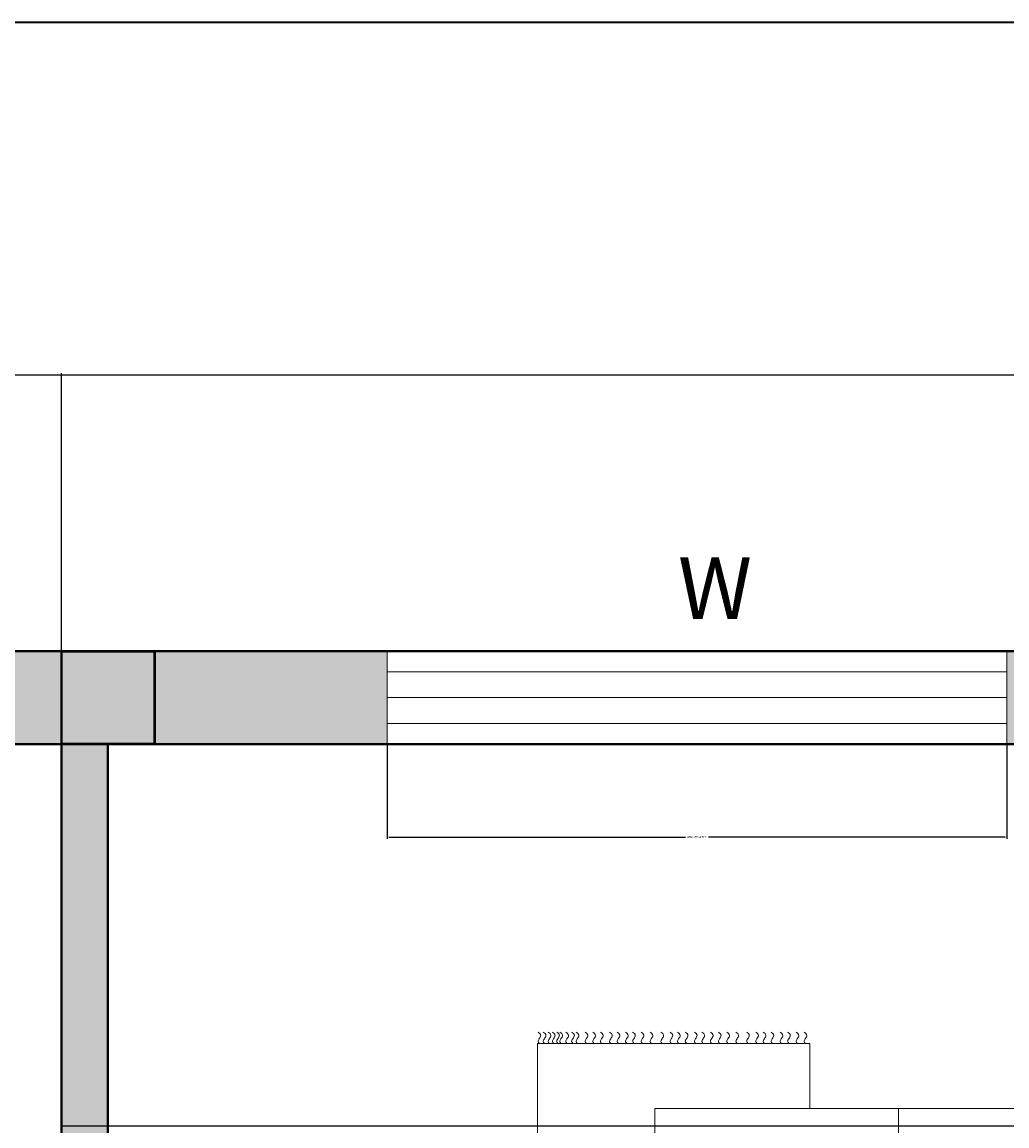
# Model space of a CAD drawing. Units: inches. Extents: x 25176543 to 25177243, y 80295576 to 80296086.
# Tile 10 of 11: x 25177000 to 25177096, y 80295979 to 80296086. Entities that reach past the tile are written whole.
import ezdxf

# ---------------------------------------------------------------- set-up
doc = ezdxf.new("R2010")
doc.units = ezdxf.units.IN
doc.header["$MEASUREMENT"] = 0
for name, color, linetype, lineweight in [('A-ANNO-DIMS', 2, 'Continuous', 18), ('A-ANNO-IDEN', 7, 'Continuous', 18), ('A-ANNO-TTLB', 7, 'Continuous', 35), ('A-COLS', 7, 'Continuous', 50), ('A-COLS-PATT', 251, 'Continuous', 13), ('A-GLAZ', 4, 'Continuous', 18), ('A-WALL', 7, 'Continuous', 40), ('A-WALL-PATT', 146, 'Continuous', 13), ('furniture', 31, 'Continuous', 13)]:
    doc.layers.add(name, color=color, linetype=linetype, lineweight=lineweight)
doc.styles.get("Standard").update_dxf_attribs({"font": 'arial.ttf'})
doc.dimstyles.get("Standard").update_dxf_attribs({"dimtxt": 0.18, "dimasz": 0.18, "dimexe": 0.18, "dimexo": 0.0625, "dimgap": 0.09, "dimtad": 0, "dimtih": 1, "dimtoh": 1, "dimdec": 4, "dimzin": 0, "dimdsep": 46, "dimtxsty": 'Standard', "dimcen": 0.09, "dimadec": 0, "dimazin": 0, "dimtfac": 1, "dimtdec": 4, "dimtofl": 0, "dimtmove": 0, "dimatfit": 3, "dimfxl": 1, "dimtolj": 1, "dimtzin": 0, "dimarcsym": 0})

# ---------------------------------------------------------------- blocks, each defined once
blk = doc.blocks.new('BED-DOUBLE-WITH-NIGHTSTANDS')
for p, q in [((5.6, 61.62), (5.6, 51.56)), ((63.65, 61.72), (63.65, 51.66)), ((68.68, 56.69), (58.62, 56.69)), ((10.63, 56.59), (0.57, 56.59)), ((49.39, 52.82), (10.63, 52.82)), ((49.39, 52.82), (58, 46.47)), ((49.44, 52.82), (49.44, 46.47)), ((49.44, 52), (10.63, 52)), ((49.44, 46.47), (58, 46.47)), ((58.05, 34.96), (10.63, 34.96)), ((4.35, 0), (4.35, 26.37)), ((4.35, 26.37), (10.65, 26.37)), ((58.05, 26.37), (67.59, 26.37)), ((67.59, 26.37), (67.59, 0)), ((67.59, 0), (4.35, 0))]:
    blk.add_line(p, q)
for points in [[(0, 50.39), (10.63, 50.5), (10.63, 62.68), (0, 62.58)], [(58.05, 62.68), (58.05, 11.37), (10.63, 11.37), (10.63, 62.68)], [(58.05, 50.5), (68.68, 50.6), (68.68, 62.78), (58.05, 62.68)], [(29.88, 59.98), (29.88, 52.82), (15.98, 52.82), (15.98, 59.98)], [(49.44, 59.98), (49.44, 52.82), (35.55, 52.82), (35.55, 59.98)]]:
    blk.add_lwpolyline(points, close=True)
for centre in [(5.6, 56.59), (63.65, 56.69)]:
    blk.add_circle(centre, 3.92)
for points, knots in [([(3.23, 25.84), (3.32, 25.96), (3.52, 26.2), (3.86, 25.96), (4.14, 25.78), (4.29, 25.89), (4.35, 25.94)], [0, 0, 0, 0, 0.400747, 0.791423, 1.067667, 1.29709, 1.29709, 1.29709, 1.29709]), ([(68.71, 25.84), (68.61, 25.96), (68.42, 26.2), (68.08, 25.96), (67.8, 25.78), (67.65, 25.89), (67.58, 25.94)], [0, 0, 0, 0, 0.400747, 0.791423, 1.067667, 1.29709, 1.29709, 1.29709, 1.29709]), ([(3.23, 25.06), (3.32, 25.18), (3.52, 25.42), (3.86, 25.18), (4.14, 25.01), (4.29, 25.11), (4.35, 25.16)], [0, 0, 0, 0, 0.400747, 0.791423, 1.067667, 1.29709, 1.29709, 1.29709, 1.29709]), ([(68.71, 25.06), (68.61, 25.18), (68.42, 25.42), (68.08, 25.18), (67.8, 25.01), (67.65, 25.11), (67.58, 25.16)], [0, 0, 0, 0, 0.400747, 0.791423, 1.067667, 1.29709, 1.29709, 1.29709, 1.29709]), ([(3.23, 24.24), (3.32, 24.36), (3.52, 24.6), (3.86, 24.36), (4.14, 24.19), (4.29, 24.3), (4.35, 24.34)], [0, 0, 0, 0, 0.400747, 0.791423, 1.067667, 1.29709, 1.29709, 1.29709, 1.29709]), ([(3.23, 23.51), (3.32, 23.63), (3.52, 23.87), (3.86, 23.63), (4.14, 23.46), (4.29, 23.57), (4.35, 23.62)], [0, 0, 0, 0, 0.400747, 0.791423, 1.067667, 1.29709, 1.29709, 1.29709, 1.29709]), ([(68.71, 24.24), (68.61, 24.36), (68.42, 24.6), (68.08, 24.36), (67.8, 24.19), (67.65, 24.3), (67.58, 24.34)], [0, 0, 0, 0, 0.400747, 0.791423, 1.067667, 1.29709, 1.29709, 1.29709, 1.29709]), ([(68.71, 23.51), (68.61, 23.63), (68.42, 23.87), (68.08, 23.63), (67.8, 23.46), (67.65, 23.57), (67.58, 23.62)], [0, 0, 0, 0, 0.400747, 0.791423, 1.067667, 1.29709, 1.29709, 1.29709, 1.29709]), ([(3.23, 22.63), (3.32, 22.75), (3.52, 22.99), (3.86, 22.75), (4.14, 22.58), (4.29, 22.69), (4.35, 22.73)], [0, 0, 0, 0, 0.400747, 0.791423, 1.067667, 1.29709, 1.29709, 1.29709, 1.29709]), ([(68.71, 22.63), (68.61, 22.75), (68.42, 22.99), (68.08, 22.75), (67.8, 22.58), (67.65, 22.69), (67.58, 22.73)], [0, 0, 0, 0, 0.400747, 0.791423, 1.067667, 1.29709, 1.29709, 1.29709, 1.29709]), ([(3.23, 21.88), (3.32, 22), (3.52, 22.24), (3.86, 22), (4.14, 21.83), (4.29, 21.93), (4.35, 21.98)], [0, 0, 0, 0, 0.400747, 0.791423, 1.067667, 1.29709, 1.29709, 1.29709, 1.29709]), ([(3.23, 21.15), (3.32, 21.27), (3.52, 21.51), (3.86, 21.27), (4.14, 21.1), (4.29, 21.21), (4.35, 21.25)], [0, 0, 0, 0, 0.400747, 0.791423, 1.067667, 1.29709, 1.29709, 1.29709, 1.29709]), ([(68.71, 21.88), (68.61, 22), (68.42, 22.24), (68.08, 22), (67.8, 21.83), (67.65, 21.93), (67.58, 21.98)], [0, 0, 0, 0, 0.400747, 0.791423, 1.067667, 1.29709, 1.29709, 1.29709, 1.29709]), ([(68.71, 21.15), (68.61, 21.27), (68.42, 21.51), (68.08, 21.27), (67.8, 21.1), (67.65, 21.21), (67.58, 21.25)], [0, 0, 0, 0, 0.400747, 0.791423, 1.067667, 1.29709, 1.29709, 1.29709, 1.29709]), ([(3.23, 20.27), (3.32, 20.39), (3.52, 20.63), (3.86, 20.39), (4.14, 20.22), (4.29, 20.32), (4.35, 20.37)], [0, 0, 0, 0, 0.400747, 0.791423, 1.067667, 1.29709, 1.29709, 1.29709, 1.29709]), ([(68.71, 20.27), (68.61, 20.39), (68.42, 20.63), (68.08, 20.39), (67.8, 20.22), (67.65, 20.32), (67.58, 20.37)], [0, 0, 0, 0, 0.400747, 0.791423, 1.067667, 1.29709, 1.29709, 1.29709, 1.29709]), ([(3.23, 19.23), (3.32, 19.35), (3.52, 19.59), (3.86, 19.35), (4.14, 19.18), (4.29, 19.29), (4.35, 19.33)], [0, 0, 0, 0, 0.400747, 0.791423, 1.067667, 1.29709, 1.29709, 1.29709, 1.29709]), ([(68.71, 19.23), (68.61, 19.35), (68.42, 19.59), (68.08, 19.35), (67.8, 19.18), (67.65, 19.29), (67.58, 19.33)], [0, 0, 0, 0, 0.400747, 0.791423, 1.067667, 1.29709, 1.29709, 1.29709, 1.29709]), ([(3.23, 18.35), (3.32, 18.47), (3.52, 18.71), (3.86, 18.47), (4.14, 18.3), (4.29, 18.4), (4.35, 18.45)], [0, 0, 0, 0, 0.400747, 0.791423, 1.067667, 1.29709, 1.29709, 1.29709, 1.29709]), ([(68.71, 18.35), (68.61, 18.47), (68.42, 18.71), (68.08, 18.47), (67.8, 18.3), (67.65, 18.4), (67.58, 18.45)], [0, 0, 0, 0, 0.400747, 0.791423, 1.067667, 1.29709, 1.29709, 1.29709, 1.29709]), ([(3.23, 17.53), (3.32, 17.65), (3.52, 17.89), (3.86, 17.65), (4.14, 17.48), (4.29, 17.59), (4.35, 17.64)], [0, 0, 0, 0, 0.400747, 0.791423, 1.067667, 1.29709, 1.29709, 1.29709, 1.29709]), ([(68.71, 17.53), (68.61, 17.65), (68.42, 17.89), (68.08, 17.65), (67.8, 17.48), (67.65, 17.59), (67.58, 17.64)], [0, 0, 0, 0, 0.400747, 0.791423, 1.067667, 1.29709, 1.29709, 1.29709, 1.29709]), ([(3.23, 16.76), (3.32, 16.88), (3.52, 17.12), (3.86, 16.88), (4.14, 16.7), (4.29, 16.81), (4.35, 16.86)], [0, 0, 0, 0, 0.400747, 0.791423, 1.067667, 1.29709, 1.29709, 1.29709, 1.29709]), ([(3.23, 15.94), (3.32, 16.06), (3.52, 16.3), (3.86, 16.06), (4.14, 15.89), (4.29, 16), (4.35, 16.04)], [0, 0, 0, 0, 0.400747, 0.791423, 1.067667, 1.29709, 1.29709, 1.29709, 1.29709]), ([(68.71, 16.76), (68.61, 16.88), (68.42, 17.12), (68.08, 16.88), (67.8, 16.7), (67.65, 16.81), (67.58, 16.86)], [0, 0, 0, 0, 0.400747, 0.791423, 1.067667, 1.29709, 1.29709, 1.29709, 1.29709]), ([(68.71, 15.94), (68.61, 16.06), (68.42, 16.3), (68.08, 16.06), (67.8, 15.89), (67.65, 16), (67.58, 16.04)], [0, 0, 0, 0, 0.400747, 0.791423, 1.067667, 1.29709, 1.29709, 1.29709, 1.29709]), ([(3.23, 15.21), (3.32, 15.33), (3.52, 15.57), (3.86, 15.33), (4.14, 15.16), (4.29, 15.27), (4.35, 15.32)], [0, 0, 0, 0, 0.400747, 0.791423, 1.067667, 1.29709, 1.29709, 1.29709, 1.29709]), ([(68.71, 15.21), (68.61, 15.33), (68.42, 15.57), (68.08, 15.33), (67.8, 15.16), (67.65, 15.27), (67.58, 15.32)], [0, 0, 0, 0, 0.400747, 0.791423, 1.067667, 1.29709, 1.29709, 1.29709, 1.29709]), ([(3.23, 14.33), (3.32, 14.45), (3.52, 14.69), (3.86, 14.45), (4.14, 14.28), (4.29, 14.38), (4.35, 14.43)], [0, 0, 0, 0, 0.400747, 0.791423, 1.067667, 1.29709, 1.29709, 1.29709, 1.29709]), ([(68.71, 14.33), (68.61, 14.45), (68.42, 14.69), (68.08, 14.45), (67.8, 14.28), (67.65, 14.38), (67.58, 14.43)], [0, 0, 0, 0, 0.400747, 0.791423, 1.067667, 1.29709, 1.29709, 1.29709, 1.29709]), ([(3.23, 13.58), (3.32, 13.7), (3.52, 13.94), (3.86, 13.7), (4.14, 13.53), (4.29, 13.63), (4.35, 13.68)], [0, 0, 0, 0, 0.400747, 0.791423, 1.067667, 1.29709, 1.29709, 1.29709, 1.29709]), ([(3.23, 12.85), (3.32, 12.97), (3.52, 13.21), (3.86, 12.97), (4.14, 12.8), (4.29, 12.9), (4.35, 12.95)], [0, 0, 0, 0, 0.400747, 0.791423, 1.067667, 1.29709, 1.29709, 1.29709, 1.29709]), ([(68.71, 13.58), (68.61, 13.7), (68.42, 13.94), (68.08, 13.7), (67.8, 13.53), (67.65, 13.63), (67.58, 13.68)], [0, 0, 0, 0, 0.400747, 0.791423, 1.067667, 1.29709, 1.29709, 1.29709, 1.29709]), ([(68.71, 12.85), (68.61, 12.97), (68.42, 13.21), (68.08, 12.97), (67.8, 12.8), (67.65, 12.9), (67.58, 12.95)], [0, 0, 0, 0, 0.400747, 0.791423, 1.067667, 1.29709, 1.29709, 1.29709, 1.29709]), ([(3.23, 11.97), (3.32, 12.09), (3.52, 12.33), (3.86, 12.09), (4.14, 11.92), (4.29, 12.02), (4.35, 12.07)], [0, 0, 0, 0, 0.400747, 0.791423, 1.067667, 1.29709, 1.29709, 1.29709, 1.29709]), ([(68.71, 11.97), (68.61, 12.09), (68.42, 12.33), (68.08, 12.09), (67.8, 11.92), (67.65, 12.02), (67.58, 12.07)], [0, 0, 0, 0, 0.400747, 0.791423, 1.067667, 1.29709, 1.29709, 1.29709, 1.29709]), ([(3.23, 10.93), (3.32, 11.05), (3.52, 11.29), (3.86, 11.05), (4.14, 10.88), (4.29, 10.99), (4.35, 11.03)], [0, 0, 0, 0, 0.400747, 0.791423, 1.067667, 1.29709, 1.29709, 1.29709, 1.29709]), ([(68.71, 10.93), (68.61, 11.05), (68.42, 11.29), (68.08, 11.05), (67.8, 10.88), (67.65, 10.99), (67.58, 11.03)], [0, 0, 0, 0, 0.400747, 0.791423, 1.067667, 1.29709, 1.29709, 1.29709, 1.29709]), ([(3.23, 10.05), (3.32, 10.17), (3.52, 10.41), (3.86, 10.17), (4.14, 10), (4.29, 10.1), (4.35, 10.15)], [0, 0, 0, 0, 0.400747, 0.791423, 1.067667, 1.29709, 1.29709, 1.29709, 1.29709]), ([(68.71, 10.05), (68.61, 10.17), (68.42, 10.41), (68.08, 10.17), (67.8, 10), (67.65, 10.1), (67.58, 10.15)], [0, 0, 0, 0, 0.400747, 0.791423, 1.067667, 1.29709, 1.29709, 1.29709, 1.29709]), ([(3.23, 9.23), (3.32, 9.35), (3.52, 9.59), (3.86, 9.35), (4.14, 9.18), (4.29, 9.29), (4.35, 9.34)], [0, 0, 0, 0, 0.400747, 0.791423, 1.067667, 1.29709, 1.29709, 1.29709, 1.29709]), ([(3.23, 8.54), (3.32, 8.66), (3.52, 8.9), (3.86, 8.66), (4.14, 8.49), (4.29, 8.6), (4.35, 8.65)], [0, 0, 0, 0, 0.400747, 0.791423, 1.067667, 1.29709, 1.29709, 1.29709, 1.29709]), ([(68.71, 9.23), (68.61, 9.35), (68.42, 9.59), (68.08, 9.35), (67.8, 9.18), (67.65, 9.29), (67.58, 9.34)], [0, 0, 0, 0, 0.400747, 0.791423, 1.067667, 1.29709, 1.29709, 1.29709, 1.29709]), ([(68.71, 8.54), (68.61, 8.66), (68.42, 8.9), (68.08, 8.66), (67.8, 8.49), (67.65, 8.6), (67.58, 8.65)], [0, 0, 0, 0, 0.400747, 0.791423, 1.067667, 1.29709, 1.29709, 1.29709, 1.29709]), ([(3.23, 7.73), (3.32, 7.85), (3.52, 8.09), (3.86, 7.85), (4.14, 7.68), (4.29, 7.78), (4.35, 7.83)], [0, 0, 0, 0, 0.400747, 0.791423, 1.067667, 1.29709, 1.29709, 1.29709, 1.29709]), ([(68.71, 7.73), (68.61, 7.85), (68.42, 8.09), (68.08, 7.85), (67.8, 7.68), (67.65, 7.78), (67.58, 7.83)], [0, 0, 0, 0, 0.400747, 0.791423, 1.067667, 1.29709, 1.29709, 1.29709, 1.29709]), ([(3.23, 7), (3.32, 7.12), (3.52, 7.36), (3.86, 7.12), (4.14, 6.95), (4.29, 7.05), (4.35, 7.1)], [0, 0, 0, 0, 0.400747, 0.791423, 1.067667, 1.29709, 1.29709, 1.29709, 1.29709]), ([(68.71, 7), (68.61, 7.12), (68.42, 7.36), (68.08, 7.12), (67.8, 6.95), (67.65, 7.05), (67.58, 7.1)], [0, 0, 0, 0, 0.400747, 0.791423, 1.067667, 1.29709, 1.29709, 1.29709, 1.29709]), ([(3.23, 6.12), (3.32, 6.24), (3.52, 6.48), (3.86, 6.24), (4.14, 6.07), (4.29, 6.17), (4.35, 6.22)], [0, 0, 0, 0, 0.400747, 0.791423, 1.067667, 1.29709, 1.29709, 1.29709, 1.29709]), ([(3.23, 5.36), (3.32, 5.49), (3.52, 5.73), (3.86, 5.49), (4.14, 5.31), (4.29, 5.42), (4.35, 5.47)], [0, 0, 0, 0, 0.400747, 0.791423, 1.067667, 1.29709, 1.29709, 1.29709, 1.29709]), ([(68.71, 6.12), (68.61, 6.24), (68.42, 6.48), (68.08, 6.24), (67.8, 6.07), (67.65, 6.17), (67.58, 6.22)], [0, 0, 0, 0, 0.400747, 0.791423, 1.067667, 1.29709, 1.29709, 1.29709, 1.29709]), ([(68.71, 5.36), (68.61, 5.49), (68.42, 5.73), (68.08, 5.49), (67.8, 5.31), (67.65, 5.42), (67.58, 5.47)], [0, 0, 0, 0, 0.400747, 0.791423, 1.067667, 1.29709, 1.29709, 1.29709, 1.29709]), ([(3.23, 4.64), (3.32, 4.76), (3.52, 5), (3.86, 4.76), (4.14, 4.59), (4.29, 4.69), (4.35, 4.74)], [0, 0, 0, 0, 0.400747, 0.791423, 1.067667, 1.29709, 1.29709, 1.29709, 1.29709]), ([(68.71, 4.64), (68.61, 4.76), (68.42, 5), (68.08, 4.76), (67.8, 4.59), (67.66, 4.69), (67.59, 4.73)], [0, 0, 0, 0, 0.400747, 0.791423, 1.067667, 1.283686, 1.283686, 1.283686, 1.283686]), ([(3.23, 3.75), (3.32, 3.88), (3.52, 4.12), (3.86, 3.88), (4.14, 3.7), (4.29, 3.81), (4.35, 3.86)], [0, 0, 0, 0, 0.400747, 0.791423, 1.067667, 1.29709, 1.29709, 1.29709, 1.29709]), ([(3.23, 3.33), (3.32, 3.45), (3.52, 3.7), (3.86, 3.44), (4.14, 3.27), (4.29, 3.38), (4.35, 3.43)], [0, 0, 0, 0, 0.407265, 0.802015, 1.07826, 1.307683, 1.307683, 1.307683, 1.307683]), ([(68.71, 3.75), (68.61, 3.88), (68.42, 4.11), (68.08, 3.88), (67.8, 3.7), (67.66, 3.81), (67.59, 3.85)], [0, 0, 0, 0, 0.400747, 0.791423, 1.067667, 1.283686, 1.283686, 1.283686, 1.283686]), ([(68.71, 3.33), (68.61, 3.45), (68.42, 3.69), (68.08, 3.45), (67.8, 3.27), (67.66, 3.38), (67.59, 3.42)], [0, 0, 0, 0, 0.402903, 0.794912, 1.071156, 1.287177, 1.287177, 1.287177, 1.287177]), ([(3.23, 2.76), (3.32, 2.88), (3.52, 3.12), (3.86, 2.88), (4.14, 2.71), (4.29, 2.81), (4.35, 2.86)], [0, 0, 0, 0, 0.400747, 0.791423, 1.067667, 1.29709, 1.29709, 1.29709, 1.29709]), ([(3.23, 2.18), (3.32, 2.31), (3.52, 2.55), (3.86, 2.31), (4.14, 2.13), (4.29, 2.24), (4.35, 2.29)], [0, 0, 0, 0, 0.400747, 0.791423, 1.067667, 1.29709, 1.29709, 1.29709, 1.29709]), ([(3.23, 1.88), (3.32, 2), (3.52, 2.24), (3.86, 2), (4.14, 1.82), (4.29, 1.93), (4.35, 1.98)], [0, 0, 0, 0, 0.400747, 0.791423, 1.067667, 1.29709, 1.29709, 1.29709, 1.29709]), ([(68.71, 2.73), (68.61, 2.85), (68.42, 3.09), (68.08, 2.85), (67.8, 2.68), (67.66, 2.78), (67.59, 2.82)], [0, 0, 0, 0, 0.400747, 0.791423, 1.067667, 1.283686, 1.283686, 1.283686, 1.283686]), ([(68.71, 2.16), (68.61, 2.28), (68.42, 2.52), (68.08, 2.28), (67.8, 2.11), (67.66, 2.21), (67.59, 2.25)], [0, 0, 0, 0, 0.400747, 0.791423, 1.067667, 1.283686, 1.283686, 1.283686, 1.283686]), ([(3.23, 1.46), (3.32, 1.58), (3.52, 1.82), (3.86, 1.58), (4.14, 1.41), (4.29, 1.51), (4.35, 1.56)], [0, 0, 0, 0, 0.400747, 0.791423, 1.067667, 1.29709, 1.29709, 1.29709, 1.29709]), ([(3.23, 1.06), (3.32, 1.18), (3.52, 1.42), (3.86, 1.18), (4.14, 1.01), (4.29, 1.11), (4.35, 1.16)], [0, 0, 0, 0, 0.400747, 0.791423, 1.067667, 1.29709, 1.29709, 1.29709, 1.29709]), ([(68.71, 1.43), (68.61, 1.55), (68.42, 1.79), (68.08, 1.55), (67.8, 1.38), (67.65, 1.48), (67.58, 1.53)], [0, 0, 0, 0, 0.400747, 0.791423, 1.067667, 1.29709, 1.29709, 1.29709, 1.29709]), ([(68.71, 1.03), (68.61, 1.15), (68.42, 1.39), (68.08, 1.15), (67.8, 0.98), (67.65, 1.09), (67.58, 1.13)], [0, 0, 0, 0, 0.400747, 0.791423, 1.067667, 1.29709, 1.29709, 1.29709, 1.29709]), ([(68.71, 1.85), (68.61, 1.97), (68.42, 2.21), (68.08, 1.97), (67.8, 1.8), (67.66, 1.9), (67.59, 1.94)], [0, 0, 0, 0, 0.400747, 0.791423, 1.067667, 1.283686, 1.283686, 1.283686, 1.283686]), ([(3.23, 0.57), (3.32, 0.7), (3.52, 0.94), (3.86, 0.7), (4.14, 0.52), (4.29, 0.63), (4.35, 0.68)], [0, 0, 0, 0, 0.400747, 0.791423, 1.067667, 1.29709, 1.29709, 1.29709, 1.29709]), ([(3.23, 0.07), (3.32, 0.19), (3.52, 0.43), (3.86, 0.19), (4.14, 0.02), (4.29, 0.13), (4.35, 0.18)], [0, 0, 0, 0, 0.400747, 0.791423, 1.067667, 1.29709, 1.29709, 1.29709, 1.29709]), ([(68.71, 0.55), (68.61, 0.67), (68.42, 0.91), (68.08, 0.67), (67.8, 0.49), (67.65, 0.6), (67.58, 0.65)], [0, 0, 0, 0, 0.400747, 0.791423, 1.067667, 1.29709, 1.29709, 1.29709, 1.29709]), ([(68.71, 0.07), (68.61, 0.19), (68.42, 0.43), (68.08, 0.19), (67.8, 0.02), (67.65, 0.13), (67.58, 0.18)], [0, 0, 0, 0, 0.400747, 0.791423, 1.067667, 1.29709, 1.29709, 1.29709, 1.29709])]:
    blk.add_open_spline(points, degree=3, knots=knots)
blk = doc.blocks.new('WIN-60IN')
for p, q in [((0, 9), (0, 0)), ((60, 9), (0, 9)), ((0, 9), (0, 4.5)), ((60, 0), (60, 9)), ((60, 7), (0, 7)), ((0, 4.5), (60, 4.5)), ((0, 2), (60, 2)), ((0, 0), (60, 0))]:
    blk.add_line(p, q)
blk = doc.blocks.new('*D20')
at = {"layer": 'A-ANNO-DIMS', "color": 0, "lineweight": -2, "transparency": 16777216}
for p, q in [((25177035.84, 80296016.24), (25177035.84, 80296007.12)), ((25177095.84, 80296016.24), (25177095.84, 80296007.12)), ((25177036.02, 80296007.3), (25177064.73, 80296007.3)), ((25177095.66, 80296007.3), (25177066.96, 80296007.3))]:
    blk.add_line(p, q, dxfattribs=at)
at = {"layer": 'A-ANNO-DIMS', "color": 0, "transparency": 16777216}
for points in [[(25177036.02, 80296007.33), (25177036.02, 80296007.27), (25177035.84, 80296007.3)], [(25177095.66, 80296007.33), (25177095.66, 80296007.27), (25177095.84, 80296007.3)]]:
    blk.add_solid(points, dxfattribs=at)
at = {"layer": 'Defpoints', "color": 0, "transparency": 16777216}
for p in [(25177035.84, 80296016.3), (25177095.84, 80296016.3), (25177095.84, 80296007.3)]:
    blk.add_point(p, dxfattribs=at)
at = {"layer": 'A-ANNO-DIMS', "color": 0, "transparency": 16777216, "insert": (25177065.84, 80296007.3), "char_height": 0.18, "attachment_point": 5}
blk.add_mtext('\\A1;WINDOW 60 TYP.', dxfattribs=at)
blk = doc.blocks.new('*D21')
at = {"layer": 'A-ANNO-DIMS', "color": 0, "lineweight": -2, "transparency": 16777216}
for p, q in [((25177095.91, 80296025.3), (25177105.02, 80296025.3)), ((25177104.84, 80296025.12), (25177104.84, 80296020.98)), ((25177104.84, 80296016.48), (25177104.84, 80296020.62)), ((25177095.91, 80296016.3), (25177105.02, 80296016.3))]:
    blk.add_line(p, q, dxfattribs=at)
at = {"layer": 'A-ANNO-DIMS', "color": 0, "transparency": 16777216}
for points in [[(25177104.81, 80296025.12), (25177104.87, 80296025.12), (25177104.84, 80296025.3)], [(25177104.81, 80296016.48), (25177104.87, 80296016.48), (25177104.84, 80296016.3)]]:
    blk.add_solid(points, dxfattribs=at)
at = {"layer": 'Defpoints', "color": 0, "transparency": 16777216}
for p in [(25177095.84, 80296025.3), (25177104.84, 80296025.3), (25177095.84, 80296016.3)]:
    blk.add_point(p, dxfattribs=at)
at = {"layer": 'A-ANNO-DIMS', "color": 0, "transparency": 16777216, "insert": (25177104.84, 80296020.8), "char_height": 0.18, "attachment_point": 5}
blk.add_mtext('\\A1;9 TYP.', dxfattribs=at)
blk = doc.blocks.new('*D48')
at = {"layer": 'A-ANNO-DIMS', "color": 0, "lineweight": -2, "transparency": 16777216}
for p, q in [((25176625.3, 80295890.36), (25176625.3, 80296052.23)), ((25177125.8, 80296025.36), (25177125.8, 80296052.23)), ((25176625.48, 80296052.05), (25176875.16, 80296052.05)), ((25177125.62, 80296052.05), (25176875.95, 80296052.05))]:
    blk.add_line(p, q, dxfattribs=at)
at = {"layer": 'A-ANNO-DIMS', "color": 0, "transparency": 16777216}
for points in [[(25176625.48, 80296052.08), (25176625.48, 80296052.02), (25176625.3, 80296052.05)], [(25177125.62, 80296052.08), (25177125.62, 80296052.02), (25177125.8, 80296052.05)]]:
    blk.add_solid(points, dxfattribs=at)
at = {"layer": 'Defpoints', "color": 0, "transparency": 16777216}
for p in [(25177125.8, 80296052.05), (25177125.8, 80296025.3), (25176625.3, 80295890.3)]:
    blk.add_point(p, dxfattribs=at)
at = {"layer": 'A-ANNO-DIMS', "color": 0, "transparency": 16777216, "insert": (25176875.55, 80296052.05), "char_height": 0.18, "attachment_point": 5}
blk.add_mtext('\\A1;500.5', dxfattribs=at)
blk = doc.blocks.new('*D66')
at = {"layer": 'A-ANNO-DIMS', "color": 0, "lineweight": -2, "transparency": 16777216}
for p, q in [((25176986.71, 80296025.36), (25176986.71, 80296052.23)), ((25177004.3, 80296025.36), (25177004.3, 80296052.23)), ((25176986.89, 80296052.05), (25176995.05, 80296052.05)), ((25177004.12, 80296052.05), (25176995.96, 80296052.05))]:
    blk.add_line(p, q, dxfattribs=at)
at = {"layer": 'A-ANNO-DIMS', "color": 0, "transparency": 16777216}
for points in [[(25176986.89, 80296052.08), (25176986.89, 80296052.02), (25176986.71, 80296052.05)], [(25177004.12, 80296052.08), (25177004.12, 80296052.02), (25177004.3, 80296052.05)]]:
    blk.add_solid(points, dxfattribs=at)
at = {"layer": 'Defpoints', "color": 0, "transparency": 16777216}
for p in [(25177004.3, 80296052.05), (25176986.71, 80296025.3), (25177004.3, 80296025.3)]:
    blk.add_point(p, dxfattribs=at)
at = {"layer": 'A-ANNO-DIMS', "color": 0, "transparency": 16777216, "insert": (25176995.51, 80296052.05), "char_height": 0.18, "attachment_point": 5}
blk.add_mtext('\\A1;17.587', dxfattribs=at)
blk = doc.blocks.new('*D70')
at = {"layer": 'A-ANNO-DIMS', "color": 0, "lineweight": -2, "transparency": 16777216}
for p, q in [((25177004.36, 80296016.3), (25177152.73, 80296016.3)), ((25177152.55, 80296016.12), (25177152.55, 80295997.99)), ((25177152.55, 80295979.5), (25177152.55, 80295997.63)), ((25177004.36, 80295979.32), (25177152.73, 80295979.32))]:
    blk.add_line(p, q, dxfattribs=at)
at = {"layer": 'A-ANNO-DIMS', "color": 0, "transparency": 16777216}
for points in [[(25177152.52, 80296016.12), (25177152.58, 80296016.12), (25177152.55, 80296016.3)], [(25177152.52, 80295979.5), (25177152.58, 80295979.5), (25177152.55, 80295979.32)]]:
    blk.add_solid(points, dxfattribs=at)
at = {"layer": 'Defpoints', "color": 0, "transparency": 16777216}
for p in [(25177004.3, 80296016.3), (25177152.55, 80296016.3), (25177004.3, 80295979.32)]:
    blk.add_point(p, dxfattribs=at)
at = {"layer": 'A-ANNO-DIMS', "color": 0, "transparency": 16777216, "insert": (25177152.55, 80295997.81), "char_height": 0.18, "attachment_point": 5}
blk.add_mtext('\\A1;36.98', dxfattribs=at)

msp = doc.modelspace()

# ---------------------------------------------------------------- hatches: boundary and pattern name
at = {"layer": 'A-COLS-PATT'}
h = msp.add_hatch(color=256, dxfattribs=at)
h.dxf.hatch_style = 1
h.paths.add_polyline_path([(25176658.8016, 80296025.3022), (25176649.8016, 80296025.3022), (25176649.8016, 80296016.3022), (25176658.8016, 80296016.3022)])
h.paths.add_polyline_path([(25176819.3016, 80296025.3022), (25176810.3016, 80296025.3022), (25176810.3016, 80296016.3022), (25176819.3016, 80296016.3022)])
h.paths.add_polyline_path([(25176876.3016, 80296025.3022), (25176867.3016, 80296025.3022), (25176867.3016, 80296016.3022), (25176876.3016, 80296016.3022)])
h.paths.add_polyline_path([(25177013.3016, 80296025.3022), (25177004.3016, 80296025.3022), (25177004.3016, 80296016.3022), (25177013.3016, 80296016.3022)])
h.paths.add_polyline_path([(25176819.3016, 80295890.3022), (25176810.3016, 80295890.3022), (25176810.3016, 80295881.3022), (25176819.3016, 80295881.3022)])
h.paths.add_polyline_path([(25176658.8016, 80295890.3022), (25176649.8016, 80295890.3022), (25176649.8016, 80295881.3022), (25176658.8016, 80295881.3022)])
h.paths.add_polyline_path([(25177125.8016, 80296025.3022), (25177116.8016, 80296025.3022), (25177116.8016, 80296016.3022), (25177125.8016, 80296016.3022)])
h.paths.add_polyline_path([(25177125.8016, 80295848.3022), (25177116.8016, 80295848.3022), (25177116.8016, 80295839.3022), (25177125.8016, 80295839.3022)])
h.paths.add_polyline_path([(25177013.3016, 80295848.3022), (25177004.3016, 80295848.3022), (25177004.3016, 80295839.3022), (25177013.3016, 80295839.3022)])
h.paths.add_polyline_path([(25177125.8016, 80295676.8022), (25177116.8016, 80295676.8022), (25177116.8016, 80295667.8022), (25177125.8016, 80295667.8022)])
h.paths.add_polyline_path([(25177013.3016, 80295676.8022), (25177004.3016, 80295676.8022), (25177004.3016, 80295667.8022), (25177013.3016, 80295667.8022)])
h.paths.add_polyline_path([(25176842.3016, 80295676.8022), (25176833.3016, 80295676.8022), (25176833.3016, 80295667.8022), (25176842.3016, 80295667.8022)])
h.paths.add_polyline_path([(25176893.3016, 80295676.8022), (25176884.3016, 80295676.8022), (25176884.3016, 80295667.8022), (25176893.3016, 80295667.8022)])
h.paths.add_polyline_path([(25176842.3016, 80295807.3022), (25176833.3016, 80295807.3022), (25176833.3016, 80295798.3022), (25176842.3016, 80295798.3022)])
h.paths.add_polyline_path([(25176658.8016, 80295807.3022), (25176649.8016, 80295807.3022), (25176649.8016, 80295798.3022), (25176658.8016, 80295798.3022)])
h.paths.add_polyline_path([(25176658.8016, 80295676.8022), (25176649.8016, 80295676.8022), (25176649.8016, 80295667.8022), (25176658.8016, 80295667.8022)])
at = {"layer": 'A-WALL-PATT'}
h = msp.add_hatch(color=256, dxfattribs=at)
h.dxf.hatch_style = 1
h.paths.add_polyline_path([(25176695.189, 80296025.3022), (25176658.8016, 80296025.3022), (25176658.8016, 80296016.3022), (25176695.189, 80296016.3022)])
h.paths.add_polyline_path([(25176810.3016, 80296025.3022), (25176755.189, 80296025.3022), (25176755.189, 80296016.3022), (25176810.3016, 80296016.3022)])
h.paths.add_polyline_path([(25176819.3016, 80296016.3022), (25176814.8016, 80296016.3022), (25176814.8016, 80295965.3022), (25176819.3016, 80295965.3022)], flags=17)
h.paths.add_polyline_path([(25176828.0421, 80296025.3022), (25176819.3016, 80296025.3022), (25176819.3016, 80296016.3022), (25176828.0421, 80296016.3022)])
h.paths.add_polyline_path([(25176867.3016, 80296025.3022), (25176852.0421, 80296025.3022), (25176852.0421, 80296016.3022), (25176867.3016, 80296016.3022)])
h.paths.add_polyline_path([(25176885.1873, 80296025.3022), (25176876.3016, 80296025.3022), (25176876.3016, 80296016.3022), (25176885.1873, 80296016.3022)])
h.paths.add_polyline_path([(25176919.8016, 80296025.3022), (25176909.1873, 80296025.3022), (25176909.1873, 80296016.3022), (25176919.8016, 80296016.3022)])
h.paths.add_polyline_path([(25176924.3016, 80296016.3022), (25176919.8016, 80296016.3022), (25176919.8016, 80295890.3022), (25176904.8016, 80295890.3022), (25176904.8016, 80295885.8022), (25176967.3016, 80295885.8022), (25176967.3016, 80295890.3022), (25176924.3016, 80295890.3022)])
h.paths.add_polyline_path([(25176924.3016, 80296025.3022), (25176919.8016, 80296025.3022), (25176919.8016, 80296016.3022), (25176924.3016, 80296016.3022)])
h.paths.add_polyline_path([(25176938.7147, 80296025.3022), (25176924.3016, 80296025.3022), (25176924.3016, 80296016.3022), (25176938.7147, 80296016.3022)])
h.paths.add_polyline_path([(25176871.8016, 80296016.3022), (25176867.3016, 80296016.3022), (25176867.3016, 80295932.3022), (25176819.3016, 80295932.3022), (25176819.3016, 80295933.3022), (25176814.8016, 80295933.3022), (25176814.8016, 80295932.3022), (25176814.8016, 80295927.3022), (25176819.3016, 80295927.3022), (25176819.3016, 80295927.8022), (25176867.3016, 80295927.8022), (25176867.3016, 80295885.8022), (25176871.8016, 80295885.8022), (25176872.8016, 80295885.8022), (25176872.8016, 80295890.3022), (25176871.8016, 80295890.3022)])
h.paths.add_polyline_path([(25177004.3016, 80296025.3022), (25176986.7147, 80296025.3022), (25176986.7147, 80296016.3022), (25177004.3016, 80296016.3022)])
h.paths.add_polyline_path([(25177035.845, 80296025.3022), (25177013.3016, 80296025.3022), (25177013.3016, 80296016.3022), (25177035.845, 80296016.3022)])
h.paths.add_polyline_path([(25177008.8016, 80296016.3022), (25177004.3016, 80296016.3022), (25177004.3016, 80295890.3022), (25177003.3016, 80295890.3022), (25177003.3016, 80295885.8022), (25177004.3016, 80295885.8022), (25177004.3016, 80295885.3022), (25177008.8016, 80295885.3022)])
h.paths.add_polyline_path([(25177116.8016, 80296025.3022), (25177095.845, 80296025.3022), (25177095.845, 80296016.3022), (25177116.8016, 80296016.3022)])
h.paths.add_polyline_path([(25177125.8016, 80296016.3022), (25177116.8016, 80296016.3022), (25177116.8016, 80295971.1334), (25177121.3016, 80295971.1334), (25177125.8016, 80295971.1334)])
h.paths.add_polyline_path([(25177116.8016, 80295848.3022), (25177013.3016, 80295848.3022), (25177013.3016, 80295843.8022), (25177116.8016, 80295843.8022)])
h.paths.add_polyline_path([(25177125.8016, 80295911.1334), (25177116.8016, 80295911.1334), (25177116.8016, 80295848.3022), (25177125.8016, 80295848.3022)])
h.paths.add_polyline_path([(25177008.8016, 80295802.3022), (25177004.3016, 80295802.3022), (25177004.3016, 80295676.8022), (25177008.8016, 80295676.8022)])
h.paths.add_polyline_path([(25176658.8016, 80295705.5694), (25176649.8016, 80295705.5694), (25176649.8016, 80295676.8022), (25176658.8016, 80295676.8022)])
h.paths.add_polyline_path([(25176658.8016, 80295798.3022), (25176649.8016, 80295798.3022), (25176649.8016, 80295765.5694), (25176654.3016, 80295765.5694), (25176658.8016, 80295765.5694)])
h.paths.add_polyline_path([(25176833.3016, 80295807.3022), (25176658.8016, 80295807.3022), (25176658.8016, 80295802.8022), (25176833.3016, 80295802.8022)])
h.paths.add_polyline_path([(25176842.3016, 80295761.3022), (25176837.8016, 80295761.3022), (25176837.8016, 80295676.8022), (25176842.3016, 80295676.8022)])
h.paths.add_polyline_path([(25176649.8016, 80295807.3022), (25176629.8016, 80295807.3022), (25176629.8016, 80295885.8022), (25176649.8016, 80295885.8022), (25176649.8016, 80295890.3022), (25176625.3016, 80295890.3022), (25176625.3016, 80295802.8022), (25176649.8016, 80295802.8022)])
h.paths.add_polyline_path([(25176810.3016, 80295890.3022), (25176658.8016, 80295890.3022), (25176658.8016, 80295885.8022), (25176810.3016, 80295885.8022)])
h.paths.add_polyline_path([(25176658.8016, 80295922.9263), (25176649.8016, 80295922.9263), (25176649.8016, 80295890.3022), (25176658.8016, 80295890.3022)])
h.paths.add_polyline_path([(25176658.8016, 80296016.3022), (25176649.8016, 80296016.3022), (25176649.8016, 80295982.9263), (25176654.3016, 80295982.9263), (25176658.8016, 80295982.9263)])

# ---------------------------------------------------------------- linework, layer by layer
at = {"layer": 'A-ANNO-TTLB'}
msp.add_lwpolyline([(25176542.8973, 80296086.2335), (25177242.9194, 80296086.2335), (25177242.9194, 80295575.9501), (25176542.8973, 80295575.9501)], close=True, dxfattribs=at)
at = {"layer": 'A-COLS'}
for p, q in [((25177004.3016, 80296025.3022), (25177013.3016, 80296025.3022)), ((25177013.3016, 80296025.3022), (25177013.3016, 80296016.3022)), ((25177013.3016, 80296016.3022), (25177004.3016, 80296016.3022))]:
    msp.add_line(p, q, dxfattribs=at)
at = {"layer": 'A-WALL'}
for p, q in [((25176649.8016, 80296025.3022), (25177125.8016, 80296025.3022)), ((25177004.3016, 80296025.3022), (25177004.3016, 80295890.3022)), ((25176649.8016, 80296016.3022), (25177125.8016, 80296016.3022)), ((25177008.8016, 80296016.3022), (25177008.8016, 80295885.3022))]:
    msp.add_line(p, q, dxfattribs=at)

# ---------------------------------------------------------------- block references
at = {"layer": 'A-GLAZ'}
msp.add_blockref('WIN-60IN', (25177035.8449, 80296016.302), dxfattribs=at)
at = {"layer": 'furniture', "rotation": 269.9999999743436}
msp.add_blockref('BED-DOUBLE-WITH-NIGHTSTANDS', (25177050.3784, 80295991.6444), dxfattribs=at)

# ---------------------------------------------------------------- texts
at = {"layer": 'A-ANNO-IDEN', "insert": (25177063.9858, 80296034.4049), "char_height": 6, "attachment_point": 1}
msp.add_mtext_dynamic_manual_height_columns('W', width=24.139595, gutter_width=1, heights=[0], dxfattribs=at)

# ---------------------------------------------------------------- dimensions: what is measured, and where the dimension line sits
at = {"layer": 'A-ANNO-DIMS'}
for base, p1, p2, override, picture, middle in [((25177125.8016, 80296052.0522), (25176625.3016, 80295890.3022), (25177125.8016, 80296025.3022), {"dimdec": 1, "dimlfac": 1, "dimrnd": 0, "dimzin": 0, "dimdsep": 46, "dimlunit": 2}, '*D48', (25176875.5516, 80296052.0522)), ((25177004.3016, 80296052.0522), (25176986.7147, 80296025.3022), (25177004.3016, 80296025.3022), {"dimdec": 3, "dimlfac": 1, "dimrnd": 0, "dimzin": 0, "dimdsep": 46, "dimlunit": 2}, '*D66', (25176995.5081, 80296052.0522))]:
    dim = msp.add_linear_dim(base=base, p1=p1, p2=p2, dimstyle='Standard', override=override, dxfattribs=at)
    dim.commit()
    dim.dimension.update_dxf_attribs({"geometry": picture, "text_midpoint": middle})
dim = msp.add_linear_dim(base=(25177104.845, 80296025.3022), p1=(25177095.845, 80296016.3022), p2=(25177095.845, 80296025.3022), angle=90, text='<> TYP.', dimstyle='Standard', override={"dimdec": 0, "dimlfac": 1, "dimrnd": 0, "dimzin": 0, "dimdsep": 46, "dimlunit": 2}, dxfattribs=at)
dim.commit()
dim.dimension.update_dxf_attribs({"geometry": '*D21', "text_midpoint": (25177104.845, 80296020.8022)})
dim = msp.add_linear_dim(base=(25177152.5516, 80296016.3022), p1=(25177004.3016, 80295979.3235), p2=(25177004.3016, 80296016.3022), angle=90, dimstyle='Standard', override={"dimdec": 2, "dimlfac": 1, "dimrnd": 0, "dimzin": 0, "dimdsep": 46, "dimlunit": 2}, dxfattribs=at)
dim.commit()
dim.dimension.update_dxf_attribs({"geometry": '*D70', "text_midpoint": (25177152.5516, 80295997.8129)})
dim = msp.add_linear_dim(base=(25177095.845, 80296007.3022), p1=(25177035.845, 80296016.3022), p2=(25177095.845, 80296016.3022), text='WINDOW <> TYP.', dimstyle='Standard', override={"dimdec": 0, "dimlfac": 1, "dimrnd": 0, "dimzin": 0, "dimdsep": 46, "dimlunit": 2}, dxfattribs=at)
dim.commit()
dim.dimension.update_dxf_attribs({"geometry": '*D20', "text_midpoint": (25177065.845, 80296007.3022)})

doc.saveas('drawing.dxf')
